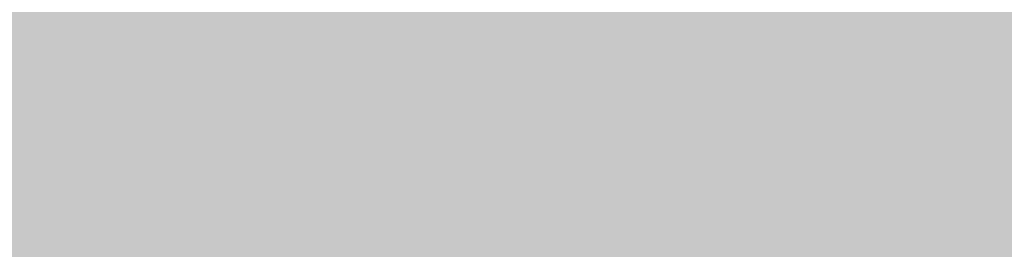
# Model space of a CAD drawing. Units: millimetres. Extents: x 0 to 2267, y 0 to 1823.
# Tile 175 of 256: x 1833.606 to 1838.83, y 1128.496 to 1129.713. Entities that reach past the tile are written whole.
import ezdxf

# ---------------------------------------------------------------- set-up
doc = ezdxf.new("R2010")
doc.units = ezdxf.units.MM
doc.header["$MEASUREMENT"] = 0
doc.layers.add('M-HATC', color=252, linetype='Continuous', lineweight=18)

msp = doc.modelspace()

# ---------------------------------------------------------------- hatches: boundary and pattern name
at = {"layer": 'M-HATC'}
h = msp.add_hatch(color=256, dxfattribs=at)
h.dxf.hatch_style = 1
h.paths.add_polyline_path([(2055.771, 1603.062), (1381.0868, 1603.062), (1381.0868, 1598.062), (2055.771, 1598.062)])
h.paths.add_polyline_path([(2055.771, 1598.062), (1381.0868, 1598.062), (1381.0868, 1593.062), (2055.771, 1593.062)])
h.paths.add_polyline_path([(2051.3074, 1536.7609), (1385.5504, 1536.7609), (1385.5504, 1526.7609), (1387.5504, 1526.7609), (1388.5366, 1525.0528), (1385.3319, 1521.2335), (1385.3319, 1521.2226), (2050.2542, 1522.7491), (2048.3212, 1525.0528), (2049.3074, 1526.7609), (2051.3074, 1526.7609)])
edge = h.paths.add_edge_path()
edge.add_arc((1847.5345, 1379.1492), 135, 222.603061, 222.890851, ccw=False)
edge.add_line((1748.1663, 1287.7656), (1683.0921, 1287.7656))
edge.add_arc((1583.7239, 1379.1492), 135, 317.109149, 317.396939, ccw=False)
edge.add_arc((1678.9686, 1290.6707), 5, 222.8909, 317.1091, ccw=False)
edge.add_arc((1774.2133, 1379.1492), 135, 222.603061, 222.890851, ccw=False)
edge.add_line((1674.8451, 1287.7656), (1609.7709, 1287.7656))
edge.add_arc((1510.4027, 1379.1492), 135, 317.109149, 317.396939, ccw=False)
edge.add_arc((1605.6474, 1290.6707), 5, 222.8909, 317.1091, ccw=False)
edge.add_arc((1700.8921, 1379.1492), 135, 222.603061, 222.890851, ccw=False)
edge.add_line((1601.5239, 1287.7656), (1536.4497, 1287.7656))
edge.add_arc((1437.0815, 1379.1492), 135, 317.109149, 317.396939, ccw=False)
edge.add_arc((1532.3262, 1290.6707), 5, 222.8909, 317.1091, ccw=False)
edge.add_arc((1627.5709, 1379.1492), 135, 222.603061, 222.890851, ccw=False)
edge.add_line((1528.2027, 1287.7656), (1505.9289, 1287.7656))
edge.add_spline(control_points=[(1505.9289, 1287.7656), (1504.2622, 1287.7656), (1504.2622, 1282.7656), (1505.9289, 1282.7656)], knot_values=[0, 0, 0, 0, 5, 5, 5, 5], degree=3, periodic=0)
edge.add_line((1505.9289, 1282.7656), (1930.9289, 1282.7656))
edge.add_spline(control_points=[(1930.9289, 1282.7656), (1932.5956, 1282.7656), (1932.5956, 1287.7656), (1930.9289, 1287.7656)], knot_values=[0, 0, 0, 0, 5, 5, 5, 5], degree=3, periodic=0)
edge.add_line((1930.9289, 1287.7656), (1903.0557, 1287.7656))
edge.add_arc((1803.6875, 1379.1492), 135, 317.109149, 317.396939, ccw=False)
edge.add_arc((1898.9322, 1290.6707), 5, 222.8909, 317.1091, ccw=False)
edge.add_arc((1994.1769, 1379.1492), 135, 222.603061, 222.890851, ccw=False)
edge.add_line((1894.8087, 1287.7656), (1829.7345, 1287.7656))
edge.add_arc((1730.3663, 1379.1492), 135, 317.109149, 317.396939, ccw=False)
edge.add_arc((1825.611, 1290.6707), 5, 222.8909, 317.1091, ccw=False)
edge.add_arc((1920.8557, 1379.1492), 135, 222.603061, 222.890851, ccw=False)
edge.add_line((1821.4875, 1287.7656), (1756.4133, 1287.7656))
edge.add_arc((1657.0451, 1379.1492), 135, 317.109149, 317.396939, ccw=False)
edge.add_arc((1752.2898, 1290.6707), 5, 222.8909, 317.1091, ccw=False)
edge = h.paths.add_edge_path()
edge.add_spline(control_points=[(1843.4289, 1227.2475), (1845.0956, 1227.2475), (1845.0956, 1232.2475), (1843.4289, 1232.2475)], knot_values=[0, 0, 0, 0, 5, 5, 5, 5], degree=3, periodic=0)
edge.add_line((1843.4289, 1232.2475), (1593.4289, 1232.2475))
edge.add_spline(control_points=[(1593.4289, 1232.2475), (1591.7622, 1232.2475), (1591.7622, 1227.2475), (1593.4289, 1227.2475)], knot_values=[0, 0, 0, 0, 5, 5, 5, 5], degree=3, periodic=0)
edge.add_line((1593.4289, 1227.2475), (1843.4289, 1227.2475))
h.paths.add_polyline_path([(1905.9289, 1127.4171), (1530.9289, 1127.4171, 0.414214), (1520.9289, 1117.4171), (1530.9289, 1117.4171), (1915.9289, 1117.4171, 0.414214)])
edge = h.paths.add_edge_path()
edge.add_arc((1397.0858, 1498.4078), 12.7299, 90.78215, 190.87871, ccw=False)
edge.add_line((1396.912, 1511.1365), (1428.0097, 1511.3488))
edge.add_line((1428.0097, 1511.3488), (1433.0097, 1511.3488))
edge.add_line((1433.0097, 1511.3488), (1434.439, 1511.3488))
edge.add_arc((1419.474, 1498.0804), 20, 41.561, 74.08211)
edge.add_line((1424.9592, 1517.3135), (1399.9351, 1517.2561))
edge.add_spline(control_points=[(1399.9307, 1517.2561), (1399.884, 1517.2131), (1399.8328, 1517.1689), (1399.7774, 1517.1236)], knot_values=[11.567499, 11.567499, 11.567499, 11.567499, 11.814249, 11.814249, 11.814249, 11.814249], degree=3, periodic=0)
edge.add_spline(control_points=[(1399.6328, 1517.0099), (1399.5831, 1516.9721), (1399.5307, 1516.9338), (1399.4759, 1516.8947)], knot_values=[11.167718, 11.167718, 11.167718, 11.167718, 11.365188, 11.365188, 11.365188, 11.365188], degree=3, periodic=0)
edge.add_spline(control_points=[(1399.3398, 1516.8001), (1399.1514, 1516.6719), (1398.9384, 1516.5377), (1398.704, 1516.3994)], knot_values=[10.376405, 10.376405, 10.376405, 10.376405, 11.00994, 11.00994, 11.00994, 11.00994], degree=3, periodic=0)
edge.add_spline(control_points=[(1398.6572, 1516.3719), (1398.5789, 1516.326), (1398.4983, 1516.2797), (1398.4155, 1516.2331)], knot_values=[10.125175, 10.125175, 10.125175, 10.125175, 10.334406, 10.334406, 10.334406, 10.334406], degree=3, periodic=0)
edge.add_spline(control_points=[(1398.2642, 1516.1487), (1398.196, 1516.1111), (1398.1263, 1516.0732), (1398.0555, 1516.0351)], knot_values=[9.832246, 9.832246, 9.832246, 9.832246, 9.999658, 9.999658, 9.999658, 9.999658], degree=3, periodic=0)
edge.add_spline(control_points=[(1397.9987, 1516.0048), (1397.7312, 1515.8621), (1397.446, 1515.7171), (1397.1466, 1515.5714)], knot_values=[9.161808, 9.161808, 9.161808, 9.161808, 9.787769, 9.787769, 9.787769, 9.787769], degree=3, periodic=0)
edge.add_spline(control_points=[(1397.1466, 1515.5714), (1396.8418, 1515.423), (1396.5222, 1515.274), (1396.1914, 1515.1262)], knot_values=[8.524455, 8.524455, 8.524455, 8.524455, 9.161808, 9.161808, 9.161808, 9.161808], degree=3, periodic=0)
edge.add_spline(control_points=[(1396.0777, 1515.0756), (1395.9854, 1515.0348), (1395.8922, 1514.994), (1395.7983, 1514.9534)], knot_values=[8.275193, 8.275193, 8.275193, 8.275193, 8.451726, 8.451726, 8.451726, 8.451726], degree=3, periodic=0)
edge.add_spline(control_points=[(1395.6018, 1514.8691), (1395.4997, 1514.8257), (1395.3968, 1514.7824), (1395.2932, 1514.7394)], knot_values=[7.962917, 7.962917, 7.962917, 7.962917, 8.152764, 8.152764, 8.152764, 8.152764], degree=3, periodic=0)
edge.add_spline(control_points=[(1395.2116, 1514.7057), (1394.8278, 1514.5475), (1394.4345, 1514.3929), (1394.0364, 1514.2442)], knot_values=[7.21254, 7.21254, 7.21254, 7.21254, 7.913148, 7.913148, 7.913148, 7.913148], degree=3, periodic=0)
edge.add_spline(control_points=[(1394.0364, 1514.2442), (1393.7076, 1514.1214), (1393.3754, 1514.0027), (1393.0427, 1513.8895)], knot_values=[6.633733, 6.633733, 6.633733, 6.633733, 7.21254, 7.21254, 7.21254, 7.21254], degree=3, periodic=0)
edge.add_spline(control_points=[(1392.8214, 1513.815), (1392.7198, 1513.7812), (1392.6181, 1513.7479), (1392.5166, 1513.7152)], knot_values=[6.328796, 6.328796, 6.328796, 6.328796, 6.505493, 6.505493, 6.505493, 6.505493], degree=3, periodic=0)
edge.add_spline(control_points=[(1392.5166, 1513.7152), (1392.3187, 1513.6515), (1392.1212, 1513.59), (1391.9244, 1513.531)], knot_values=[5.984605, 5.984605, 5.984605, 5.984605, 6.328796, 6.328796, 6.328796, 6.328796], degree=3, periodic=0)
edge.add_spline(control_points=[(1391.7915, 1513.4915), (1391.3122, 1513.3501), (1390.8384, 1513.2239), (1390.3784, 1513.1171)], knot_values=[5.066697, 5.066697, 5.066697, 5.066697, 5.907055, 5.907055, 5.907055, 5.907055], degree=3, periodic=0)
edge.add_spline(control_points=[(1390.3784, 1513.1171), (1390.1797, 1513.071), (1389.9836, 1513.0284), (1389.7907, 1512.9899)], knot_values=[4.70367, 4.70367, 4.70367, 4.70367, 5.066695, 5.066695, 5.066695, 5.066695], degree=3, periodic=0)
edge.add_spline(control_points=[(1389.422, 1512.9204), (1389.2459, 1512.8892), (1389.0729, 1512.8617), (1388.9036, 1512.8381)], knot_values=[4.130571, 4.130571, 4.130571, 4.130571, 4.469816, 4.469816, 4.469816, 4.469816], degree=3, periodic=0)
edge.add_spline(control_points=[(1388.9036, 1512.8381), (1388.591, 1512.7946), (1388.2911, 1512.7644), (1388.0071, 1512.7494)], knot_values=[3.504031, 3.504031, 3.504031, 3.504031, 4.130571, 4.130571, 4.130571, 4.130571], degree=3, periodic=0)
edge.add_spline(control_points=[(1387.9356, 1512.7459), (1387.8538, 1512.7423), (1387.7733, 1512.74), (1387.6944, 1512.739)], knot_values=[3.268866, 3.268866, 3.268866, 3.268866, 3.451164, 3.451164, 3.451164, 3.451164], degree=3, periodic=0)
edge.add_spline(control_points=[(1387.3351, 1512.7443), (1387.2076, 1512.7499), (1387.0847, 1512.7597), (1386.967, 1512.7739)], knot_values=[2.670686, 2.670686, 2.670686, 2.670686, 2.984, 2.984, 2.984, 2.984], degree=3, periodic=0)
edge.add_spline(control_points=[(1386.8327, 1512.7922), (1386.8209, 1512.7941), (1386.8092, 1512.7959), (1386.7975, 1512.7979)], knot_values=[2.516981, 2.516981, 2.516981, 2.516981, 2.549528, 2.549528, 2.549528, 2.549528], degree=3, periodic=0)
edge.add_spline(control_points=[(1386.4526, 1512.8735), (1386.4257, 1512.881), (1386.3993, 1512.889), (1386.3733, 1512.8972)], knot_values=[2.095869, 2.095869, 2.095869, 2.095869, 2.17941, 2.17941, 2.17941, 2.17941], degree=3, periodic=0)
edge.add_spline(control_points=[(1386.0691, 1513.0189), (1386.0634, 1513.0217), (1386.0577, 1513.0246), (1386.052, 1513.0275)], knot_values=[1.72453, 1.72453, 1.72453, 1.72453, 1.745933, 1.745933, 1.745933, 1.745933], degree=3, periodic=0)
edge.add_arc((1399.474, 1498.0804), 20, 131.82432, 180)
edge.add_arc((1630.3336, 1505.5484), 250.9708, 181.705176, 236.427975)
edge.add_arc((1605.3399, 1483.3044), 218.7822, 238.660829, 243.34961)
edge.add_arc((1647.0911, 1510.3592), 262.8986, 183.129836, 237.853442, ccw=False)
h.paths.add_polyline_path([(1406.5369, 1391.9644, 0.149382), (1491.5506, 1296.4418, -0.129517)], flags=17)
edge = h.paths.add_edge_path()
edge.add_arc((2037.3838, 1498.0804), 20, 0, 48.26587)
edge.add_spline(control_points=[(2050.6973, 1513.0052), (2050.6512, 1512.9847), (2050.6034, 1512.9655), (2050.5539, 1512.9477)], knot_values=[1.835652, 1.835652, 1.835652, 1.835652, 2.000781, 2.000781, 2.000781, 2.000781], degree=3, periodic=0)
edge.add_spline(control_points=[(2050.4616, 1512.9166), (2050.479, 1512.9221), (2050.4963, 1512.9277), (2050.5133, 1512.9335)], knot_values=[2.045477, 2.045477, 2.045477, 2.045477, 2.101389, 2.101389, 2.101389, 2.101389], degree=3, periodic=0)
edge.add_spline(control_points=[(2050.129, 1512.8342), (2050.1984, 1512.8473), (2050.2657, 1512.8623), (2050.3308, 1512.8792)], knot_values=[2.237629, 2.237629, 2.237629, 2.237629, 2.435841, 2.435841, 2.435841, 2.435841], degree=3, periodic=0)
edge.add_spline(control_points=[(2050.0946, 1512.8278), (2050.1061, 1512.8299), (2050.1176, 1512.832), (2050.129, 1512.8342)], knot_values=[2.435841, 2.435841, 2.435841, 2.435841, 2.468321, 2.468321, 2.468321, 2.468321], degree=3, periodic=0)
edge.add_spline(control_points=[(2049.7843, 1512.7851), (2049.8552, 1512.7922), (2049.9243, 1512.8008), (2049.9917, 1512.8109)], knot_values=[2.563852, 2.563852, 2.563852, 2.563852, 2.748541, 2.748541, 2.748541, 2.748541], degree=3, periodic=0)
edge.add_spline(control_points=[(2049.4052, 1512.7617), (2049.5364, 1512.7653), (2049.6629, 1512.773), (2049.7843, 1512.7851)], knot_values=[2.748541, 2.748541, 2.748541, 2.748541, 3.064882, 3.064882, 3.064882, 3.064882], degree=3, periodic=0)
edge.add_spline(control_points=[(2049.1698, 1512.7597), (2049.2336, 1512.7591), (2049.2965, 1512.7594), (2049.3584, 1512.7606)], knot_values=[3.102309, 3.102309, 3.102309, 3.102309, 3.2503, 3.2503, 3.2503, 3.2503], degree=3, periodic=0)
edge.add_spline(control_points=[(2048.8573, 1512.7691), (2048.9638, 1512.7638), (2049.068, 1512.7606), (2049.1698, 1512.7597)], knot_values=[3.2503, 3.2503, 3.2503, 3.2503, 3.486069, 3.486069, 3.486069, 3.486069], degree=3, periodic=0)
edge.add_spline(control_points=[(2048.6924, 1512.7789), (2048.3729, 1512.8009), (2048.0345, 1512.8411), (2047.6817, 1512.897)], knot_values=[3.606429, 3.606429, 3.606429, 3.606429, 4.2989, 4.2989, 4.2989, 4.2989], degree=3, periodic=0)
edge.add_spline(control_points=[(2047.6817, 1512.897), (2047.5458, 1512.9185), (2047.4077, 1512.9424), (2047.2678, 1512.9685)], knot_values=[4.2989, 4.2989, 4.2989, 4.2989, 4.565769, 4.565769, 4.565769, 4.565769], degree=3, periodic=0)
edge.add_spline(control_points=[(2047.2678, 1512.9685), (2047.1449, 1512.9914), (2047.0207, 1513.016), (2046.8951, 1513.0422)], knot_values=[4.565769, 4.565769, 4.565769, 4.565769, 4.799971, 4.799971, 4.799971, 4.799971], degree=3, periodic=0)
edge.add_spline(control_points=[(2046.8951, 1513.0422), (2046.5286, 1513.1188), (2046.1513, 1513.209), (2045.7676, 1513.3107)], knot_values=[4.799971, 4.799971, 4.799971, 4.799971, 5.483718, 5.483718, 5.483718, 5.483718], degree=3, periodic=0)
edge.add_spline(control_points=[(2045.7676, 1513.3107), (2045.3724, 1513.4154), (2044.9704, 1513.5322), (2044.5662, 1513.6588)], knot_values=[5.483718, 5.483718, 5.483718, 5.483718, 6.187866, 6.187866, 6.187866, 6.187866], degree=3, periodic=0)
edge.add_spline(control_points=[(2044.5662, 1513.6588), (2044.4149, 1513.7061), (2044.2633, 1513.7549), (2044.1116, 1513.8048)], knot_values=[6.187866, 6.187866, 6.187866, 6.187866, 6.451551, 6.451551, 6.451551, 6.451551], degree=3, periodic=0)
edge.add_spline(control_points=[(2044.1116, 1513.8048), (2043.9967, 1513.8427), (2043.8817, 1513.8813), (2043.7668, 1513.9205)], knot_values=[6.451551, 6.451551, 6.451551, 6.451551, 6.651434, 6.651434, 6.651434, 6.651434], degree=3, periodic=0)
edge.add_spline(control_points=[(2043.7668, 1513.9205), (2043.3716, 1514.0554), (2042.9774, 1514.1979), (2042.5886, 1514.3458)], knot_values=[6.651434, 6.651434, 6.651434, 6.651434, 7.338879, 7.338879, 7.338879, 7.338879], degree=3, periodic=0)
edge.add_spline(control_points=[(2042.5886, 1514.3458), (2042.1643, 1514.5071), (2041.7465, 1514.6749), (2041.3409, 1514.846)], knot_values=[7.338879, 7.338879, 7.338879, 7.338879, 8.089209, 8.089209, 8.089209, 8.089209], degree=3, periodic=0)
edge.add_spline(control_points=[(2041.3409, 1514.846), (2041.1028, 1514.9465), (2040.869, 1515.0481), (2040.6405, 1515.1502)], knot_values=[8.089209, 8.089209, 8.089209, 8.089209, 8.529587, 8.529587, 8.529587, 8.529587], degree=3, periodic=0)
edge.add_spline(control_points=[(2040.51, 1515.2089), (2040.0824, 1515.4022), (2039.6747, 1515.5971), (2039.295, 1515.7894)], knot_values=[8.613818, 8.613818, 8.613818, 8.613818, 9.44571, 9.44571, 9.44571, 9.44571], degree=3, periodic=0)
edge.add_spline(control_points=[(2039.295, 1515.7894), (2039.0618, 1515.9075), (2038.8391, 1516.0246), (2038.6288, 1516.1398)], knot_values=[9.44571, 9.44571, 9.44571, 9.44571, 9.956404, 9.956404, 9.956404, 9.956404], degree=3, periodic=0)
edge.add_spline(control_points=[(2038.6288, 1516.1398), (2038.5187, 1516.2001), (2038.4121, 1516.2598), (2038.309, 1516.3189)], knot_values=[9.956404, 9.956404, 9.956404, 9.956404, 10.223542, 10.223542, 10.223542, 10.223542], degree=3, periodic=0)
edge.add_spline(control_points=[(2038.309, 1516.3189), (2038.2138, 1516.3735), (2038.1216, 1516.4276), (2038.0328, 1516.481)], knot_values=[10.223542, 10.223542, 10.223542, 10.223542, 10.47051, 10.47051, 10.47051, 10.47051], degree=3, periodic=0)
edge.add_spline(control_points=[(2038.0328, 1516.481), (2037.7855, 1516.6296), (2037.5639, 1516.773), (2037.3722, 1516.909)], knot_values=[10.47051, 10.47051, 10.47051, 10.47051, 11.15767, 11.15767, 11.15767, 11.15767], degree=3, periodic=0)
edge.add_spline(control_points=[(2037.3722, 1516.909), (2037.2789, 1516.9752), (2037.1927, 1517.0396), (2037.1142, 1517.102)], knot_values=[11.15767, 11.15767, 11.15767, 11.15767, 11.49227, 11.49227, 11.49227, 11.49227], degree=3, periodic=0)
edge.add_spline(control_points=[(2036.8564, 1517.3259), (2036.9148, 1517.2692), (2036.9814, 1517.2103), (2037.0557, 1517.1492)], knot_values=[11.577341, 11.577341, 11.577341, 11.577341, 11.91035, 11.91035, 11.91035, 11.91035], degree=3, periodic=0)
edge.add_spline(control_points=[(2036.8074, 1517.3748), (2036.823, 1517.3587), (2036.8393, 1517.3424), (2036.8564, 1517.3259)], knot_values=[11.91035, 11.91035, 11.91035, 11.91035, 12.007402, 12.007402, 12.007402, 12.007402], degree=3, periodic=0)
edge.add_spline(control_points=[(2036.7017, 1517.494), (2036.7104, 1517.483), (2036.7196, 1517.4719), (2036.7291, 1517.4606)], knot_values=[12.184155, 12.184155, 12.184155, 12.184155, 12.255409, 12.255409, 12.255409, 12.255409], degree=3, periodic=0)
edge.add_spline(control_points=[(2036.6159, 1517.6205), (2036.62, 1517.613), (2036.6243, 1517.6055), (2036.6289, 1517.5979)], knot_values=[12.487913, 12.487913, 12.487913, 12.487913, 12.541035, 12.541035, 12.541035, 12.541035], degree=3, periodic=0)
edge.add_spline(control_points=[(2036.5635, 1517.786), (2036.5637, 1517.7794), (2036.5642, 1517.7726), (2036.565, 1517.7658)], knot_values=[12.911761, 12.911761, 12.911761, 12.911761, 12.968286, 12.968286, 12.968286, 12.968286], degree=3, periodic=0)
edge.add_spline(control_points=[(2036.6166, 1517.9304), (2036.6125, 1517.9259), (2036.6086, 1517.9212), (2036.6049, 1517.9165)], knot_values=[13.382527, 13.382527, 13.382527, 13.382527, 13.433791, 13.433791, 13.433791, 13.433791], degree=3, periodic=0)
edge.add_spline(control_points=[(2036.749, 1518.017), (2036.7361, 1518.0116), (2036.7239, 1518.006), (2036.7124, 1518.0002)], knot_values=[13.726299, 13.726299, 13.726299, 13.726299, 13.809928, 13.809928, 13.809928, 13.809928], degree=3, periodic=0)
edge.add_spline(control_points=[(2036.8604, 1518.0528), (2036.8386, 1518.0474), (2036.8181, 1518.0416), (2036.7988, 1518.0353)], knot_values=[13.910887, 13.910887, 13.910887, 13.910887, 14.02153, 14.02153, 14.02153, 14.02153], degree=3, periodic=0)
edge.add_line((2036.9639, 1518.0804), (2032.3838, 1518.0804))
edge.add_line((2032.3838, 1518.0804), (2027.3838, 1518.0804))
edge.add_line((2027.3838, 1518.0804), (2022.3838, 1518.0804))
edge.add_line((2022.3838, 1518.0804), (2017.3838, 1518.0804))
edge.add_arc((2017.3838, 1498.0804), 20, 90, 138.439)
edge.add_line((2002.4188, 1511.3488), (2003.8481, 1511.3488))
edge.add_line((2003.8481, 1511.3488), (2008.8481, 1511.3488))
edge.add_line((2008.8481, 1511.3488), (2039.772, 1511.1377))
edge.add_arc((2039.772, 1498.4078), 12.7299, -10.87871, 90, ccw=False)
edge.add_arc((1789.7668, 1510.3592), 262.8986, 302.146558, 356.870164, ccw=False)
edge.add_arc((1831.5179, 1483.3044), 218.7822, 296.65039, 301.339171)
edge.add_arc((1806.5242, 1505.5484), 250.9708, 303.572025, 358.294824)
h.paths.add_polyline_path([(2030.321, 1391.9644, -0.129517), (1945.3072, 1296.4418, 0.149382)], flags=17)
edge = h.paths.add_edge_path()
edge.add_spline(control_points=[(2037.2464, 1518.0821), (2037.2898, 1518.081), (2037.3355, 1518.0804), (2037.3838, 1518.0804)], knot_values=[0.000012, 0.000012, 0.000012, 0.000012, 0.144754, 0.144754, 0.144754, 0.144754], degree=3, periodic=0)
edge.add_line((2037.3357, 1518.0804), (2037.0096, 1518.0804))
edge.add_spline(control_points=[(2037.0096, 1518.0804), (2036.9822, 1518.0768), (2036.956, 1518.0727), (2036.9312, 1518.0681)], knot_values=[14.13465, 14.13465, 14.13465, 14.13465, 14.247197, 14.247197, 14.247197, 14.247197], degree=3, periodic=0)
edge.add_spline(control_points=[(2036.9312, 1518.0681), (2036.9276, 1518.0674), (2036.9241, 1518.0667), (2036.9205, 1518.0661)], knot_values=[14.118315, 14.118315, 14.118315, 14.118315, 14.13465, 14.13465, 14.13465, 14.13465], degree=3, periodic=0)
edge.add_spline(control_points=[(2036.9205, 1518.0661), (2036.9118, 1518.0644), (2036.9032, 1518.0626), (2036.8948, 1518.0608)], knot_values=[14.078086, 14.078086, 14.078086, 14.078086, 14.118315, 14.118315, 14.118315, 14.118315], degree=3, periodic=0)
edge.add_spline(control_points=[(2036.8948, 1518.0608), (2036.883, 1518.0583), (2036.8716, 1518.0556), (2036.8604, 1518.0528)], knot_values=[14.02153, 14.02153, 14.02153, 14.02153, 14.078086, 14.078086, 14.078086, 14.078086], degree=3, periodic=0)
edge.add_spline(control_points=[(2036.8604, 1518.0528), (2036.8386, 1518.0474), (2036.8181, 1518.0416), (2036.7988, 1518.0353)], knot_values=[13.910887, 13.910887, 13.910887, 13.910887, 14.02153, 14.02153, 14.02153, 14.02153], degree=3, periodic=0)
edge.add_spline(control_points=[(2036.7988, 1518.0353), (2036.7981, 1518.035), (2036.7974, 1518.0348), (2036.7967, 1518.0346)], knot_values=[13.906906, 13.906906, 13.906906, 13.906906, 13.910887, 13.910887, 13.910887, 13.910887], degree=3, periodic=0)
edge.add_spline(control_points=[(2036.7967, 1518.0346), (2036.7882, 1518.0318), (2036.7799, 1518.0289), (2036.7719, 1518.0259)], knot_values=[13.857826, 13.857826, 13.857826, 13.857826, 13.906906, 13.906906, 13.906906, 13.906906], degree=3, periodic=0)
edge.add_spline(control_points=[(2036.7719, 1518.0259), (2036.764, 1518.023), (2036.7564, 1518.02), (2036.749, 1518.017)], knot_values=[13.809928, 13.809928, 13.809928, 13.809928, 13.857826, 13.857826, 13.857826, 13.857826], degree=3, periodic=0)
edge.add_spline(control_points=[(2036.749, 1518.017), (2036.7361, 1518.0116), (2036.7239, 1518.006), (2036.7124, 1518.0002)], knot_values=[13.726299, 13.726299, 13.726299, 13.726299, 13.809928, 13.809928, 13.809928, 13.809928], degree=3, periodic=0)
edge.add_spline(control_points=[(2036.7124, 1518.0002), (2036.7121, 1518), (2036.7118, 1517.9999), (2036.7115, 1517.9997)], knot_values=[13.723993, 13.723993, 13.723993, 13.723993, 13.726299, 13.726299, 13.726299, 13.726299], degree=3, periodic=0)
edge.add_spline(control_points=[(2036.7115, 1517.9997), (2036.7063, 1517.9971), (2036.7013, 1517.9944), (2036.6965, 1517.9917)], knot_values=[13.686536, 13.686536, 13.686536, 13.686536, 13.723993, 13.723993, 13.723993, 13.723993], degree=3, periodic=0)
edge.add_spline(control_points=[(2036.6965, 1517.9917), (2036.6919, 1517.9891), (2036.6874, 1517.9865), (2036.6831, 1517.9839)], knot_values=[13.651251, 13.651251, 13.651251, 13.651251, 13.686536, 13.686536, 13.686536, 13.686536], degree=3, periodic=0)
edge.add_spline(control_points=[(2036.6831, 1517.9839), (2036.6764, 1517.9798), (2036.67, 1517.9757), (2036.6639, 1517.9714)], knot_values=[13.596804, 13.596804, 13.596804, 13.596804, 13.651251, 13.651251, 13.651251, 13.651251], degree=3, periodic=0)
edge.add_spline(control_points=[(2036.6639, 1517.9714), (2036.6636, 1517.9712), (2036.6633, 1517.9709), (2036.6629, 1517.9707)], knot_values=[13.593956, 13.593956, 13.593956, 13.593956, 13.596804, 13.596804, 13.596804, 13.596804], degree=3, periodic=0)
edge.add_spline(control_points=[(2036.6629, 1517.9707), (2036.6603, 1517.9689), (2036.6577, 1517.967), (2036.6552, 1517.9651)], knot_values=[13.570322, 13.570322, 13.570322, 13.570322, 13.593956, 13.593956, 13.593956, 13.593956], degree=3, periodic=0)
edge.add_spline(control_points=[(2036.6552, 1517.9651), (2036.6525, 1517.9631), (2036.6499, 1517.9611), (2036.6474, 1517.9591)], knot_values=[13.545477, 13.545477, 13.545477, 13.545477, 13.570322, 13.570322, 13.570322, 13.570322], degree=3, periodic=0)
edge.add_spline(control_points=[(2036.6474, 1517.9591), (2036.6472, 1517.9589), (2036.6471, 1517.9588), (2036.6469, 1517.9587)], knot_values=[13.543931, 13.543931, 13.543931, 13.543931, 13.545477, 13.545477, 13.545477, 13.545477], degree=3, periodic=0)
edge.add_spline(control_points=[(2036.6469, 1517.9587), (2036.6412, 1517.9541), (2036.6358, 1517.9494), (2036.6307, 1517.9447)], knot_values=[13.488237, 13.488237, 13.488237, 13.488237, 13.543931, 13.543931, 13.543931, 13.543931], degree=3, periodic=0)
edge.add_spline(control_points=[(2036.6307, 1517.9447), (2036.6282, 1517.9423), (2036.6257, 1517.9399), (2036.6233, 1517.9374)], knot_values=[13.460307, 13.460307, 13.460307, 13.460307, 13.488237, 13.488237, 13.488237, 13.488237], degree=3, periodic=0)
edge.add_spline(control_points=[(2036.6233, 1517.9374), (2036.6215, 1517.9356), (2036.6198, 1517.9338), (2036.6181, 1517.932)], knot_values=[13.439712, 13.439712, 13.439712, 13.439712, 13.460307, 13.460307, 13.460307, 13.460307], degree=3, periodic=0)
edge.add_spline(control_points=[(2036.6181, 1517.932), (2036.6176, 1517.9315), (2036.6171, 1517.9309), (2036.6166, 1517.9304)], knot_values=[13.433791, 13.433791, 13.433791, 13.433791, 13.439712, 13.439712, 13.439712, 13.439712], degree=3, periodic=0)
edge.add_spline(control_points=[(2036.6166, 1517.9304), (2036.6125, 1517.9259), (2036.6086, 1517.9212), (2036.6049, 1517.9165)], knot_values=[13.382527, 13.382527, 13.382527, 13.382527, 13.433791, 13.433791, 13.433791, 13.433791], degree=3, periodic=0)
edge.add_spline(control_points=[(2036.6049, 1517.9165), (2036.6026, 1517.9135), (2036.6004, 1517.9104), (2036.5982, 1517.9074)], knot_values=[13.350017, 13.350017, 13.350017, 13.350017, 13.382527, 13.382527, 13.382527, 13.382527], degree=3, periodic=0)
edge.add_spline(control_points=[(2036.5982, 1517.9074), (2036.5972, 1517.9059), (2036.5962, 1517.9043), (2036.5952, 1517.9028)], knot_values=[13.333922, 13.333922, 13.333922, 13.333922, 13.350017, 13.350017, 13.350017, 13.350017], degree=3, periodic=0)
edge.add_spline(control_points=[(2036.5952, 1517.9028), (2036.5945, 1517.9018), (2036.5939, 1517.9009), (2036.5933, 1517.8999)], knot_values=[13.323828, 13.323828, 13.323828, 13.323828, 13.333922, 13.333922, 13.333922, 13.333922], degree=3, periodic=0)
edge.add_spline(control_points=[(2036.5933, 1517.8999), (2036.5905, 1517.8955), (2036.5879, 1517.8909), (2036.5855, 1517.8864)], knot_values=[13.277545, 13.277545, 13.277545, 13.277545, 13.323828, 13.323828, 13.323828, 13.323828], degree=3, periodic=0)
edge.add_spline(control_points=[(2036.5855, 1517.8864), (2036.5836, 1517.8827), (2036.5817, 1517.8789), (2036.5801, 1517.8751)], knot_values=[13.240119, 13.240119, 13.240119, 13.240119, 13.277545, 13.277545, 13.277545, 13.277545], degree=3, periodic=0)
edge.add_spline(control_points=[(2036.5801, 1517.8751), (2036.5795, 1517.8739), (2036.579, 1517.8727), (2036.5785, 1517.8715)], knot_values=[13.228211, 13.228211, 13.228211, 13.228211, 13.240119, 13.240119, 13.240119, 13.240119], degree=3, periodic=0)
edge.add_spline(control_points=[(2036.5785, 1517.8715), (2036.578, 1517.8702), (2036.5774, 1517.869), (2036.5769, 1517.8677)], knot_values=[13.215717, 13.215717, 13.215717, 13.215717, 13.228211, 13.228211, 13.228211, 13.228211], degree=3, periodic=0)
edge.add_spline(control_points=[(2036.5769, 1517.8677), (2036.5755, 1517.864), (2036.5741, 1517.8603), (2036.5729, 1517.8565)], knot_values=[13.179847, 13.179847, 13.179847, 13.179847, 13.215717, 13.215717, 13.215717, 13.215717], degree=3, periodic=0)
edge.add_spline(control_points=[(2036.5729, 1517.8565), (2036.5713, 1517.8515), (2036.5699, 1517.8464), (2036.5687, 1517.8413)], knot_values=[13.132017, 13.132017, 13.132017, 13.132017, 13.179847, 13.179847, 13.179847, 13.179847], degree=3, periodic=0)
edge.add_spline(control_points=[(2036.5687, 1517.8413), (2036.5684, 1517.8402), (2036.5682, 1517.8392), (2036.568, 1517.8382)], knot_values=[13.122482, 13.122482, 13.122482, 13.122482, 13.132017, 13.132017, 13.132017, 13.132017], degree=3, periodic=0)
edge.add_spline(control_points=[(2036.568, 1517.8382), (2036.5676, 1517.8363), (2036.5672, 1517.8345), (2036.5669, 1517.8327)], knot_values=[13.105592, 13.105592, 13.105592, 13.105592, 13.122482, 13.122482, 13.122482, 13.122482], degree=3, periodic=0)
edge.add_spline(control_points=[(2036.5669, 1517.8327), (2036.5662, 1517.8292), (2036.5657, 1517.8257), (2036.5652, 1517.8222)], knot_values=[13.074063, 13.074063, 13.074063, 13.074063, 13.105592, 13.105592, 13.105592, 13.105592], degree=3, periodic=0)
edge.add_spline(control_points=[(2036.5652, 1517.8222), (2036.5652, 1517.8222), (2036.5652, 1517.8222), (2036.5652, 1517.8222)], knot_values=[13.074043, 13.074043, 13.074043, 13.074043, 13.074063, 13.074063, 13.074063, 13.074063], degree=3, periodic=0)
edge.add_spline(control_points=[(2036.5652, 1517.8222), (2036.5644, 1517.8164), (2036.5639, 1517.8106), (2036.5636, 1517.8046)], knot_values=[13.021884, 13.021884, 13.021884, 13.021884, 13.074043, 13.074043, 13.074043, 13.074043], degree=3, periodic=0)
edge.add_spline(control_points=[(2036.5636, 1517.8046), (2036.5636, 1517.804), (2036.5636, 1517.8034), (2036.5635, 1517.8028)], knot_values=[13.01674, 13.01674, 13.01674, 13.01674, 13.021884, 13.021884, 13.021884, 13.021884], degree=3, periodic=0)
edge.add_spline(control_points=[(2036.5635, 1517.8028), (2036.5634, 1517.8005), (2036.5634, 1517.7982), (2036.5634, 1517.7958)], knot_values=[12.996438, 12.996438, 12.996438, 12.996438, 13.01674, 13.01674, 13.01674, 13.01674], degree=3, periodic=0)
edge.add_spline(control_points=[(2036.5634, 1517.7958), (2036.5633, 1517.7926), (2036.5634, 1517.7893), (2036.5635, 1517.786)], knot_values=[12.968286, 12.968286, 12.968286, 12.968286, 12.996438, 12.996438, 12.996438, 12.996438], degree=3, periodic=0)
edge.add_spline(control_points=[(2036.5635, 1517.786), (2036.5637, 1517.7794), (2036.5642, 1517.7726), (2036.565, 1517.7658)], knot_values=[12.911761, 12.911761, 12.911761, 12.911761, 12.968286, 12.968286, 12.968286, 12.968286], degree=3, periodic=0)
edge.add_spline(control_points=[(2036.565, 1517.7658), (2036.565, 1517.7657), (2036.565, 1517.7656), (2036.565, 1517.7656)], knot_values=[12.911017, 12.911017, 12.911017, 12.911017, 12.911761, 12.911761, 12.911761, 12.911761], degree=3, periodic=0)
edge.add_spline(control_points=[(2036.565, 1517.7656), (2036.5654, 1517.7625), (2036.5658, 1517.7593), (2036.5663, 1517.7562)], knot_values=[12.88528, 12.88528, 12.88528, 12.88528, 12.911017, 12.911017, 12.911017, 12.911017], degree=3, periodic=0)
edge.add_spline(control_points=[(2036.5663, 1517.7562), (2036.5667, 1517.7534), (2036.5672, 1517.7506), (2036.5677, 1517.7478)], knot_values=[12.862519, 12.862519, 12.862519, 12.862519, 12.88528, 12.88528, 12.88528, 12.88528], degree=3, periodic=0)
edge.add_spline(control_points=[(2036.5677, 1517.7478), (2036.5678, 1517.7474), (2036.5679, 1517.7469), (2036.568, 1517.7465)], knot_values=[12.858885, 12.858885, 12.858885, 12.858885, 12.862519, 12.862519, 12.862519, 12.862519], degree=3, periodic=0)
edge.add_spline(control_points=[(2036.568, 1517.7465), (2036.5692, 1517.7399), (2036.5707, 1517.7332), (2036.5724, 1517.7264)], knot_values=[12.8053, 12.8053, 12.8053, 12.8053, 12.858885, 12.858885, 12.858885, 12.858885], degree=3, periodic=0)
edge.add_spline(control_points=[(2036.5724, 1517.7264), (2036.5734, 1517.7226), (2036.5745, 1517.7187), (2036.5756, 1517.7149)], knot_values=[12.775176, 12.775176, 12.775176, 12.775176, 12.8053, 12.8053, 12.8053, 12.8053], degree=3, periodic=0)
edge.add_spline(control_points=[(2036.5756, 1517.7149), (2036.5763, 1517.7125), (2036.577, 1517.7102), (2036.5778, 1517.7078)], knot_values=[12.756759, 12.756759, 12.756759, 12.756759, 12.775176, 12.775176, 12.775176, 12.775176], degree=3, periodic=0)
edge.add_spline(control_points=[(2036.5778, 1517.7078), (2036.5781, 1517.7067), (2036.5784, 1517.7057), (2036.5787, 1517.7047)], knot_values=[12.748742, 12.748742, 12.748742, 12.748742, 12.756759, 12.756759, 12.756759, 12.756759], degree=3, periodic=0)
edge.add_spline(control_points=[(2036.5787, 1517.7047), (2036.5808, 1517.6983), (2036.5831, 1517.6919), (2036.5856, 1517.6854)], knot_values=[12.69959, 12.69959, 12.69959, 12.69959, 12.748742, 12.748742, 12.748742, 12.748742], degree=3, periodic=0)
edge.add_spline(control_points=[(2036.5856, 1517.6854), (2036.5876, 1517.68), (2036.5898, 1517.6746), (2036.5921, 1517.6692)], knot_values=[12.659038, 12.659038, 12.659038, 12.659038, 12.69959, 12.69959, 12.69959, 12.69959], degree=3, periodic=0)
edge.add_spline(control_points=[(2036.5921, 1517.6692), (2036.594, 1517.6648), (2036.5959, 1517.6605), (2036.5979, 1517.6561)], knot_values=[12.626806, 12.626806, 12.626806, 12.626806, 12.659038, 12.659038, 12.659038, 12.659038], degree=3, periodic=0)
edge.add_spline(control_points=[(2036.5979, 1517.6561), (2036.5984, 1517.6551), (2036.5989, 1517.6541), (2036.5993, 1517.6531)], knot_values=[12.619394, 12.619394, 12.619394, 12.619394, 12.626806, 12.626806, 12.626806, 12.626806], degree=3, periodic=0)
edge.add_spline(control_points=[(2036.5993, 1517.6531), (2036.6043, 1517.6424), (2036.6099, 1517.6315), (2036.6159, 1517.6205)], knot_values=[12.541039, 12.541039, 12.541039, 12.541039, 12.619394, 12.619394, 12.619394, 12.619394], degree=3, periodic=0)
edge.add_spline(control_points=[(2036.6159, 1517.6205), (2036.6159, 1517.6205), (2036.6159, 1517.6205), (2036.6159, 1517.6205)], knot_values=[12.541035, 12.541035, 12.541035, 12.541035, 12.541039, 12.541039, 12.541039, 12.541039], degree=3, periodic=0)
edge.add_spline(control_points=[(2036.6159, 1517.6205), (2036.62, 1517.613), (2036.6243, 1517.6055), (2036.6289, 1517.5979)], knot_values=[12.487913, 12.487913, 12.487913, 12.487913, 12.541035, 12.541035, 12.541035, 12.541035], degree=3, periodic=0)
edge.add_spline(control_points=[(2036.6289, 1517.5979), (2036.6326, 1517.5916), (2036.6365, 1517.5853), (2036.6406, 1517.5789)], knot_values=[12.443982, 12.443982, 12.443982, 12.443982, 12.487913, 12.487913, 12.487913, 12.487913], degree=3, periodic=0)
edge.add_spline(control_points=[(2036.6406, 1517.5789), (2036.6414, 1517.5776), (2036.6423, 1517.5763), (2036.6431, 1517.5749)], knot_values=[12.434996, 12.434996, 12.434996, 12.434996, 12.443982, 12.443982, 12.443982, 12.443982], degree=3, periodic=0)
edge.add_spline(control_points=[(2036.6431, 1517.5749), (2036.6531, 1517.5596), (2036.6639, 1517.5439), (2036.6756, 1517.528)], knot_values=[12.329647, 12.329647, 12.329647, 12.329647, 12.434996, 12.434996, 12.434996, 12.434996], degree=3, periodic=0)
edge.add_spline(control_points=[(2036.6756, 1517.528), (2036.6839, 1517.5168), (2036.6925, 1517.5055), (2036.7017, 1517.494)], knot_values=[12.255409, 12.255409, 12.255409, 12.255409, 12.329647, 12.329647, 12.329647, 12.329647], degree=3, periodic=0)
edge.add_spline(control_points=[(2036.7017, 1517.494), (2036.7104, 1517.483), (2036.7196, 1517.4719), (2036.7291, 1517.4606)], knot_values=[12.184155, 12.184155, 12.184155, 12.184155, 12.255409, 12.255409, 12.255409, 12.255409], degree=3, periodic=0)
edge.add_spline(control_points=[(2036.7291, 1517.4606), (2036.7436, 1517.4435), (2036.759, 1517.4262), (2036.7753, 1517.4085)], knot_values=[12.075961, 12.075961, 12.075961, 12.075961, 12.184155, 12.184155, 12.184155, 12.184155], degree=3, periodic=0)
edge.add_spline(control_points=[(2036.7753, 1517.4085), (2036.7763, 1517.4075), (2036.7773, 1517.4064), (2036.7783, 1517.4054)], knot_values=[12.069502, 12.069502, 12.069502, 12.069502, 12.075961, 12.075961, 12.075961, 12.075961], degree=3, periodic=0)
edge.add_spline(control_points=[(2036.7783, 1517.4054), (2036.7877, 1517.3953), (2036.7974, 1517.385), (2036.8074, 1517.3748)], knot_values=[12.007402, 12.007402, 12.007402, 12.007402, 12.069502, 12.069502, 12.069502, 12.069502], degree=3, periodic=0)
edge.add_spline(control_points=[(2036.8074, 1517.3748), (2036.823, 1517.3587), (2036.8393, 1517.3424), (2036.8564, 1517.3259)], knot_values=[11.91035, 11.91035, 11.91035, 11.91035, 12.007402, 12.007402, 12.007402, 12.007402], degree=3, periodic=0)
edge.add_spline(control_points=[(2036.8564, 1517.3259), (2036.9148, 1517.2692), (2036.9814, 1517.2103), (2037.0557, 1517.1492)], knot_values=[11.577341, 11.577341, 11.577341, 11.577341, 11.91035, 11.91035, 11.91035, 11.91035], degree=3, periodic=0)
edge.add_spline(control_points=[(2037.0557, 1517.1492), (2037.0747, 1517.1336), (2037.0942, 1517.1179), (2037.1142, 1517.102)], knot_values=[11.49227, 11.49227, 11.49227, 11.49227, 11.577341, 11.577341, 11.577341, 11.577341], degree=3, periodic=0)
edge.add_spline(control_points=[(2037.1142, 1517.102), (2037.1927, 1517.0396), (2037.2789, 1516.9752), (2037.3722, 1516.909)], knot_values=[11.15767, 11.15767, 11.15767, 11.15767, 11.49227, 11.49227, 11.49227, 11.49227], degree=3, periodic=0)
edge.add_spline(control_points=[(2037.3722, 1516.909), (2037.5639, 1516.773), (2037.7855, 1516.6296), (2038.0328, 1516.481)], knot_values=[10.47051, 10.47051, 10.47051, 10.47051, 11.15767, 11.15767, 11.15767, 11.15767], degree=3, periodic=0)
edge.add_spline(control_points=[(2038.0328, 1516.481), (2038.1216, 1516.4276), (2038.2138, 1516.3735), (2038.309, 1516.3189)], knot_values=[10.223542, 10.223542, 10.223542, 10.223542, 10.47051, 10.47051, 10.47051, 10.47051], degree=3, periodic=0)
edge.add_spline(control_points=[(2038.309, 1516.3189), (2038.4121, 1516.2598), (2038.5187, 1516.2001), (2038.6288, 1516.1398)], knot_values=[9.956404, 9.956404, 9.956404, 9.956404, 10.223542, 10.223542, 10.223542, 10.223542], degree=3, periodic=0)
edge.add_spline(control_points=[(2038.6288, 1516.1398), (2038.8391, 1516.0246), (2039.0618, 1515.9075), (2039.295, 1515.7894)], knot_values=[9.44571, 9.44571, 9.44571, 9.44571, 9.956404, 9.956404, 9.956404, 9.956404], degree=3, periodic=0)
edge.add_spline(control_points=[(2039.295, 1515.7894), (2039.6747, 1515.5971), (2040.0824, 1515.4022), (2040.51, 1515.2089)], knot_values=[8.613818, 8.613818, 8.613818, 8.613818, 9.44571, 9.44571, 9.44571, 9.44571], degree=3, periodic=0)
edge.add_spline(control_points=[(2040.51, 1515.2089), (2040.5533, 1515.1893), (2040.5968, 1515.1697), (2040.6405, 1515.1502)], knot_values=[8.529587, 8.529587, 8.529587, 8.529587, 8.613818, 8.613818, 8.613818, 8.613818], degree=3, periodic=0)
edge.add_spline(control_points=[(2040.6405, 1515.1502), (2040.869, 1515.0481), (2041.1028, 1514.9465), (2041.3409, 1514.846)], knot_values=[8.089209, 8.089209, 8.089209, 8.089209, 8.529587, 8.529587, 8.529587, 8.529587], degree=3, periodic=0)
edge.add_spline(control_points=[(2041.3409, 1514.846), (2041.7465, 1514.6749), (2042.1643, 1514.5071), (2042.5886, 1514.3458)], knot_values=[7.338879, 7.338879, 7.338879, 7.338879, 8.089209, 8.089209, 8.089209, 8.089209], degree=3, periodic=0)
edge.add_spline(control_points=[(2042.5886, 1514.3458), (2042.9774, 1514.1979), (2043.3716, 1514.0554), (2043.7668, 1513.9205)], knot_values=[6.651434, 6.651434, 6.651434, 6.651434, 7.338879, 7.338879, 7.338879, 7.338879], degree=3, periodic=0)
edge.add_spline(control_points=[(2043.7668, 1513.9205), (2043.8817, 1513.8813), (2043.9967, 1513.8427), (2044.1116, 1513.8048)], knot_values=[6.451551, 6.451551, 6.451551, 6.451551, 6.651434, 6.651434, 6.651434, 6.651434], degree=3, periodic=0)
edge.add_spline(control_points=[(2044.1116, 1513.8048), (2044.2633, 1513.7549), (2044.4149, 1513.7061), (2044.5662, 1513.6588)], knot_values=[6.187866, 6.187866, 6.187866, 6.187866, 6.451551, 6.451551, 6.451551, 6.451551], degree=3, periodic=0)
edge.add_spline(control_points=[(2044.5662, 1513.6588), (2044.9704, 1513.5322), (2045.3724, 1513.4154), (2045.7676, 1513.3107)], knot_values=[5.483718, 5.483718, 5.483718, 5.483718, 6.187866, 6.187866, 6.187866, 6.187866], degree=3, periodic=0)
edge.add_spline(control_points=[(2045.7676, 1513.3107), (2046.1513, 1513.209), (2046.5286, 1513.1188), (2046.8951, 1513.0422)], knot_values=[4.799971, 4.799971, 4.799971, 4.799971, 5.483718, 5.483718, 5.483718, 5.483718], degree=3, periodic=0)
edge.add_spline(control_points=[(2046.8951, 1513.0422), (2047.0207, 1513.016), (2047.1449, 1512.9914), (2047.2678, 1512.9685)], knot_values=[4.565769, 4.565769, 4.565769, 4.565769, 4.799971, 4.799971, 4.799971, 4.799971], degree=3, periodic=0)
edge.add_spline(control_points=[(2047.2678, 1512.9685), (2047.4077, 1512.9424), (2047.5458, 1512.9185), (2047.6817, 1512.897)], knot_values=[4.2989, 4.2989, 4.2989, 4.2989, 4.565769, 4.565769, 4.565769, 4.565769], degree=3, periodic=0)
edge.add_spline(control_points=[(2047.6817, 1512.897), (2048.0345, 1512.8411), (2048.3729, 1512.8009), (2048.6924, 1512.7789)], knot_values=[3.606429, 3.606429, 3.606429, 3.606429, 4.2989, 4.2989, 4.2989, 4.2989], degree=3, periodic=0)
edge.add_spline(control_points=[(2048.6924, 1512.7789), (2048.7479, 1512.7751), (2048.8029, 1512.7718), (2048.8573, 1512.7691)], knot_values=[3.486069, 3.486069, 3.486069, 3.486069, 3.606429, 3.606429, 3.606429, 3.606429], degree=3, periodic=0)
edge.add_spline(control_points=[(2048.8573, 1512.7691), (2048.9638, 1512.7638), (2049.068, 1512.7606), (2049.1698, 1512.7597)], knot_values=[3.2503, 3.2503, 3.2503, 3.2503, 3.486069, 3.486069, 3.486069, 3.486069], degree=3, periodic=0)
edge.add_spline(control_points=[(2049.1698, 1512.7597), (2049.2336, 1512.7591), (2049.2965, 1512.7594), (2049.3584, 1512.7606)], knot_values=[3.102309, 3.102309, 3.102309, 3.102309, 3.2503, 3.2503, 3.2503, 3.2503], degree=3, periodic=0)
edge.add_spline(control_points=[(2049.3584, 1512.7606), (2049.3741, 1512.7609), (2049.3897, 1512.7613), (2049.4052, 1512.7617)], knot_values=[3.064882, 3.064882, 3.064882, 3.064882, 3.102309, 3.102309, 3.102309, 3.102309], degree=3, periodic=0)
edge.add_spline(control_points=[(2049.4052, 1512.7617), (2049.5364, 1512.7653), (2049.6629, 1512.773), (2049.7843, 1512.7851)], knot_values=[2.748541, 2.748541, 2.748541, 2.748541, 3.064882, 3.064882, 3.064882, 3.064882], degree=3, periodic=0)
edge.add_spline(control_points=[(2049.7843, 1512.7851), (2049.8552, 1512.7922), (2049.9243, 1512.8008), (2049.9917, 1512.8109)], knot_values=[2.563852, 2.563852, 2.563852, 2.563852, 2.748541, 2.748541, 2.748541, 2.748541], degree=3, periodic=0)
edge.add_spline(control_points=[(2049.9917, 1512.8109), (2050.0265, 1512.8161), (2050.0608, 1512.8218), (2050.0946, 1512.8278)], knot_values=[2.468321, 2.468321, 2.468321, 2.468321, 2.563852, 2.563852, 2.563852, 2.563852], degree=3, periodic=0)
edge.add_spline(control_points=[(2050.0946, 1512.8278), (2050.1061, 1512.8299), (2050.1176, 1512.832), (2050.129, 1512.8342)], knot_values=[2.435841, 2.435841, 2.435841, 2.435841, 2.468321, 2.468321, 2.468321, 2.468321], degree=3, periodic=0)
edge.add_spline(control_points=[(2050.129, 1512.8342), (2050.1984, 1512.8473), (2050.2657, 1512.8623), (2050.3308, 1512.8792)], knot_values=[2.237629, 2.237629, 2.237629, 2.237629, 2.435841, 2.435841, 2.435841, 2.435841], degree=3, periodic=0)
edge.add_spline(control_points=[(2050.3308, 1512.8792), (2050.3754, 1512.8908), (2050.4191, 1512.9032), (2050.4616, 1512.9166)], knot_values=[2.101389, 2.101389, 2.101389, 2.101389, 2.237629, 2.237629, 2.237629, 2.237629], degree=3, periodic=0)
edge.add_spline(control_points=[(2050.4616, 1512.9166), (2050.479, 1512.9221), (2050.4963, 1512.9277), (2050.5133, 1512.9335)], knot_values=[2.045477, 2.045477, 2.045477, 2.045477, 2.101389, 2.101389, 2.101389, 2.101389], degree=3, periodic=0)
edge.add_spline(control_points=[(2050.5133, 1512.9335), (2050.527, 1512.9382), (2050.5405, 1512.9429), (2050.5539, 1512.9477)], knot_values=[2.000781, 2.000781, 2.000781, 2.000781, 2.045477, 2.045477, 2.045477, 2.045477], degree=3, periodic=0)
edge.add_spline(control_points=[(2050.5539, 1512.9477), (2050.6034, 1512.9655), (2050.6512, 1512.9847), (2050.6973, 1513.0052)], knot_values=[1.835652, 1.835652, 1.835652, 1.835652, 2.000781, 2.000781, 2.000781, 2.000781], degree=3, periodic=0)
edge.add_arc((2037.3838, 1498.0804), 20, 48.26587, 90.12993)
edge = h.paths.add_edge_path(flags=16)
edge.add_spline(control_points=[(1386.1389, 1512.9859), (1388.92, 1511.7395), (1398.0387, 1515.5187), (1399.9307, 1517.2561)], knot_values=[1.831046, 1.831046, 1.831046, 1.831046, 11.814249, 11.814249, 11.814249, 11.814249], degree=3, periodic=0)
edge.add_line((1399.9307, 1517.2561), (1393.7435, 1517.2419))
edge.add_arc((1399.474, 1498.0804), 20, 106.6501, 131.8173)
h = msp.add_hatch(color=256, dxfattribs=at)
h.dxf.hatch_style = 1
h.paths.add_polyline_path([(2042.8886, 1580.1796), (2055.771, 1593.062), (1381.0868, 1593.062), (1393.9692, 1580.1796), (1374.086, 1560.2964), (2062.7718, 1560.2964)])
h.paths.add_polyline_path([(1843.4289, 1201.3297), (1843.4289, 1227.2475), (1593.4289, 1227.2475), (1593.4289, 1201.3297, -0.228274), (1574.5989, 1162.2346), (1530.9289, 1127.4171), (1905.9289, 1127.4171), (1862.2589, 1162.2346, -0.228274)])

doc.saveas('drawing.dxf')
